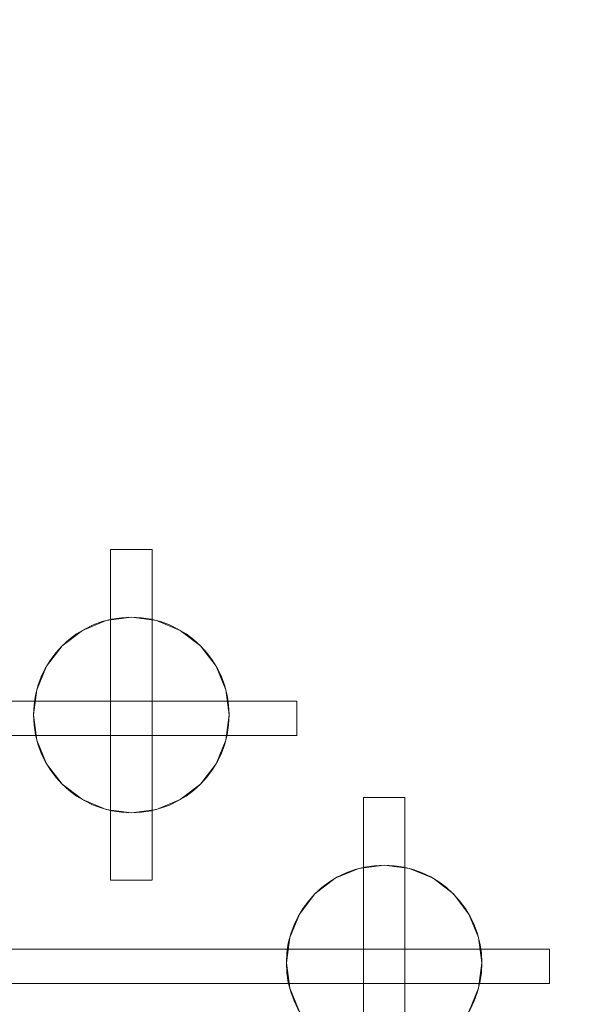
# Model space of a CAD drawing. Units: inches. Extents: x 2696 to 3240, y 1564 to 2310.
# Tile 9 of 76: x 2898.411 to 2903.397, y 1643.56 to 1652.487. Entities that reach past the tile are written whole.
import ezdxf

# ---------------------------------------------------------------- set-up
doc = ezdxf.new("R2010")
doc.units = ezdxf.units.IN
for name, color, linetype, lineweight in [('A-ANNO-DIMS', 3, 'Continuous', 18), ('A-FLOR-FIXT', 8, 'Continuous', 18), ('A-FURN', 251, 'Continuous', 13)]:
    doc.layers.add(name, color=color, linetype=linetype, lineweight=lineweight)
doc.layers.add('FURNITURE', color=250, linetype='Continuous')
doc.styles.add('TIMES NEW', font='times.ttf')
doc.dimstyles.new('Siddhuu', dxfattribs={"dimtxt": 6, "dimasz": 2.5, "dimexe": 1.25, "dimexo": 0.625, "dimtad": 1, "dimdec": 1, "dimlunit": 4, "dimtxsty": 'TIMES NEW', "dimcen": 2.5, "dimclrd": 256, "dimclre": 1, "dimclrt": 7, "dimadec": 0, "dimazin": 0, "dimtfac": 1, "dimtdec": 1, "dimtmove": 0, "dimatfit": 3, "dimfxl": 1, "dimtolj": 1, "dimlwd": -1, "dimarcsym": 0})

# ---------------------------------------------------------------- blocks, each defined once
blk = doc.blocks.new('A$C1af1f523')
at = {"layer": 'A-FURN'}
for p, q in [((-2.9003, 3.9351), (-2.9003, 0.9365)), ((-2.9003, 3.9351, 0.5), (-2.9003, 0.9365, 0.5)), ((-2.9003, 3.9351), (-2.9003, 3.9351, 0.5)), ((-2.5253, 3.9351), (-2.9003, 3.9351)), ((-2.5253, 3.9351, 0.5), (-2.9003, 3.9351, 0.5)), ((-2.5253, 3.9351), (-2.5253, 0.9365)), ((-2.5253, 3.9351, 0.5), (-2.5253, 0.9365, 0.5)), ((-2.5253, 3.9351), (-2.5253, 3.9351, 0.5)), ((-2.7128, 3.3215), (-2.7128, 3.3215, 0.5)), ((-2.9421, 3.2913), (-2.9421, 3.2913, 0.5)), ((-2.4835, 3.2913), (-2.4835, 3.2913, 0.5)), ((-3.1558, 3.2028), (-3.1558, 3.2028, 0.5)), ((-2.2698, 3.2028), (-2.2698, 3.2028, 0.5)), ((-3.3393, 3.062), (-3.3393, 3.062, 0.5)), ((-2.0863, 3.062), (-2.0863, 3.062, 0.5)), ((-3.4801, 2.8785), (-3.4801, 2.8785, 0.5)), ((-1.9455, 2.8785), (-1.9455, 2.8785, 0.5)), ((-3.5686, 2.6648), (-3.5686, 2.6648, 0.5)), ((-1.857, 2.6648), (-1.857, 2.6648, 0.5)), ((0, 2.5605), (-4.2116, 2.5605)), ((0, 2.5605, 0.5), (-4.2116, 2.5605, 0.5)), ((-4.2116, 2.5605), (-4.2116, 2.5605, 0.5)), ((-4.2116, 2.5594), (-4.2116, 2.248)), ((-4.2116, 2.5594, 0.5), (-4.2116, 2.248, 0.5)), ((-4.2116, 2.5594), (-4.2116, 2.5594, 0.5)), ((-3.5988, 2.4355), (-3.5988, 2.4355, 0.5)), ((-1.8268, 2.4355), (-1.8268, 2.4355, 0.5)), ((0, 2.248), (-4.2116, 2.248)), ((0, 2.248, 0.5), (-4.2116, 2.248, 0.5)), ((-4.2116, 2.248), (-4.2116, 2.248, 0.5)), ((-4.2116, 2.248), (-4.2116, 2.2469)), ((-4.2116, 2.248, 0.5), (-4.2116, 2.2469, 0.5)), ((-4.2116, 2.2469), (-4.2116, 2.2469, 0.5)), ((-3.5686, 2.2061), (-3.5686, 2.2061, 0.5)), ((-1.857, 2.2061), (-1.857, 2.2061, 0.5)), ((-3.4801, 1.9924), (-3.4801, 1.9924, 0.5)), ((-1.9455, 1.9924), (-1.9455, 1.9924, 0.5)), ((-3.3393, 1.8089), (-3.3393, 1.8089, 0.5)), ((-2.0863, 1.8089), (-2.0863, 1.8089, 0.5)), ((-4.8156, 1.6871), (-5.1906, 1.6871)), ((-4.8156, 1.6871, 0.5), (-5.1906, 1.6871, 0.5)), ((-5.1906, 1.6871), (-5.1906, 1.6871, 0.5)), ((-5.1906, 1.6871), (-5.1901, -1.3115)), ((-5.1906, 1.6871, 0.5), (-5.1901, -1.3115, 0.5)), ((-4.8156, 1.6871), (-4.8156, 1.6871, 0.5)), ((-4.8156, 1.6871), (-4.8151, -1.3115)), ((-4.8156, 1.6871, 0.5), (-4.8151, -1.3115, 0.5)), ((-3.1558, 1.6681), (-3.1558, 1.6681, 0.5)), ((-2.2698, 1.6681), (-2.2698, 1.6681, 0.5)), ((-2.9421, 1.5796), (-2.9421, 1.5796, 0.5)), ((-2.7128, 1.5494), (-2.7128, 1.5494, 0.5)), ((-2.4835, 1.5796), (-2.4835, 1.5796, 0.5)), ((-5.0026, 1.0735), (-5.0026, 1.0735, 0.5)), ((-5.232, 1.0433), (-5.232, 1.0433, 0.5)), ((-4.7733, 1.0433), (-4.7733, 1.0433, 0.5)), ((-5.4457, 0.9548), (-5.4457, 0.9548, 0.5)), ((-4.5596, 0.9548), (-4.5596, 0.9548, 0.5)), ((-2.9003, 0.9365), (-2.9003, 0.9365, 0.5)), ((-2.5253, 0.9365), (-2.8979, 0.9365)), ((-2.5253, 0.9365, 0.5), (-2.8979, 0.9365, 0.5)), ((-2.8979, 0.9365), (-2.8979, 0.9365, 0.5)), ((-2.5253, 0.9365), (-2.5253, 0.9365, 0.5)), ((-5.6292, 0.814), (-5.6292, 0.814, 0.5)), ((-4.3761, 0.814), (-4.3761, 0.814, 0.5)), ((-5.77, 0.6305), (-5.77, 0.6305, 0.5)), ((-4.2353, 0.6305), (-4.2353, 0.6305, 0.5)), ((-5.8585, 0.4168), (-5.8585, 0.4168, 0.5)), ((-4.1468, 0.4168), (-4.1468, 0.4168, 0.5)), ((0, 0.3125), (-6.5015, 0.3125)), ((0, 0.3125, 0.5), (-6.5015, 0.3125, 0.5)), ((-6.5015, 0.3125), (-6.5015, 0.3125, 0.5)), ((-6.5015, 0.3114), (-6.5015, 0)), ((-6.5015, 0.3114, 0.5), (-6.5015, 0, 0.5)), ((-6.5015, 0.3114), (-6.5015, 0.3114, 0.5)), ((-5.8887, 0.1875), (-5.8887, 0.1875, 0.5)), ((-4.1166, 0.1875), (-4.1166, 0.1875, 0.5)), ((0, 0), (-6.5015, 0)), ((0, 0, 0.5), (-6.5015, 0, 0.5)), ((-6.5015, 0), (-6.5015, 0, 0.5)), ((-6.5015, 0), (-6.5015, -0.0011)), ((-6.5015, 0, 0.5), (-6.5015, -0.0011, 0.5)), ((-6.5015, -0.0011), (-6.5015, -0.0011, 0.5)), ((-5.8585, -0.0418), (-5.8585, -0.0418, 0.5)), ((-4.1468, -0.0418), (-4.1468, -0.0418, 0.5)), ((-5.77, -0.2555), (-5.77, -0.2555, 0.5)), ((-4.2353, -0.2555), (-4.2353, -0.2555, 0.5)), ((-5.6292, -0.439), (-5.6292, -0.439, 0.5)), ((-4.3761, -0.439), (-4.3761, -0.439, 0.5)), ((-5.4457, -0.5798), (-5.4457, -0.5798, 0.5)), ((-4.5596, -0.5798), (-4.5596, -0.5798, 0.5)), ((-2.898, -0.5642), (-2.898, -3.5628)), ((-2.898, -0.5642, 0.5), (-2.898, -3.5628, 0.5)), ((-2.898, -0.5642), (-2.898, -0.5642, 0.5)), ((-2.523, -0.5642), (-2.898, -0.5642)), ((-2.523, -0.5642, 0.5), (-2.898, -0.5642, 0.5)), ((-2.523, -0.5642), (-2.523, -3.5628)), ((-2.523, -0.5642, 0.5), (-2.523, -3.5628, 0.5)), ((-2.523, -0.5642), (-2.523, -0.5642, 0.5)), ((-5.232, -0.6683), (-5.232, -0.6683, 0.5)), ((-5.0026, -0.6985), (-5.0026, -0.6985, 0.5)), ((-4.7733, -0.6683), (-4.7733, -0.6683, 0.5)), ((-2.9398, -1.208), (-2.9398, -1.208, 0.5)), ((-2.7105, -1.1778), (-2.7105, -1.1778, 0.5)), ((-2.4812, -1.208), (-2.4812, -1.208, 0.5)), ((-5.1901, -1.3115), (-5.1901, -1.3115, 0.5)), ((-4.8151, -1.3115), (-5.1878, -1.3115)), ((-4.8151, -1.3115, 0.5), (-5.1878, -1.3115, 0.5)), ((-5.1878, -1.3115), (-5.1878, -1.3115, 0.5)), ((-4.8151, -1.3115), (-4.8151, -1.3115, 0.5)), ((-3.1535, -1.2965), (-3.1535, -1.2965, 0.5)), ((-2.2675, -1.2965), (-2.2675, -1.2965, 0.5)), ((-3.337, -1.4373), (-3.337, -1.4373, 0.5)), ((-2.084, -1.4373), (-2.084, -1.4373, 0.5)), ((-3.4778, -1.6208), (-3.4778, -1.6208, 0.5)), ((-1.9432, -1.6208), (-1.9432, -1.6208, 0.5)), ((-3.5664, -1.8345), (-3.5664, -1.8345, 0.5)), ((-1.8547, -1.8345), (-1.8547, -1.8345, 0.5)), ((0, -1.9388), (-4.2094, -1.9388)), ((0, -1.9388, 0.5), (-4.2094, -1.9388, 0.5)), ((-4.2094, -1.9388), (-4.2094, -1.9388, 0.5)), ((-4.2094, -1.9399), (-4.2094, -2.2513)), ((-4.2094, -1.9399, 0.5), (-4.2094, -2.2513, 0.5)), ((-4.2094, -1.9399), (-4.2094, -1.9399, 0.5)), ((-3.5965, -2.0638), (-3.5965, -2.0638, 0.5)), ((-1.8245, -2.0638), (-1.8245, -2.0638, 0.5)), ((0, -2.2513), (-4.2094, -2.2513)), ((0, -2.2513, 0.5), (-4.2094, -2.2513, 0.5)), ((-4.2094, -2.2513), (-4.2094, -2.2513, 0.5)), ((-4.2094, -2.2513), (-4.2094, -2.2524)), ((-4.2094, -2.2513, 0.5), (-4.2094, -2.2524, 0.5)), ((-4.2094, -2.2524), (-4.2094, -2.2524, 0.5)), ((-3.5664, -2.2931), (-3.5664, -2.2931, 0.5)), ((-1.8547, -2.2931), (-1.8547, -2.2931, 0.5)), ((-3.4778, -2.5068), (-3.4778, -2.5068, 0.5)), ((-1.9432, -2.5068), (-1.9432, -2.5068, 0.5)), ((-3.337, -2.6903), (-3.337, -2.6903, 0.5)), ((-2.084, -2.6903), (-2.084, -2.6903, 0.5)), ((-3.1535, -2.8311), (-3.1535, -2.8311, 0.5)), ((-2.2675, -2.8311), (-2.2675, -2.8311, 0.5)), ((-2.9398, -2.9196), (-2.9398, -2.9196, 0.5)), ((-2.4812, -2.9196), (-2.4812, -2.9196, 0.5)), ((-2.7105, -2.9498), (-2.7105, -2.9498, 0.5)), ((-2.898, -3.5628), (-2.898, -3.5628, 0.5)), ((-2.523, -3.5628), (-2.8956, -3.5628)), ((-2.523, -3.5628, 0.5), (-2.8956, -3.5628, 0.5)), ((-2.8956, -3.5628), (-2.8956, -3.5628, 0.5)), ((-2.523, -3.5628), (-2.523, -3.5628, 0.5))]:
    blk.add_line(p, q, dxfattribs=at)
for centre in [(-2.7128, 2.4355), (-2.7128, 2.4355, 0.5), (-5.0026, 0.1875), (-5.0026, 0.1875, 0.5), (-2.7105, -2.0638), (-2.7105, -2.0638, 0.5)]:
    blk.add_circle(centre, 0.886, dxfattribs=at)
at = {"layer": 'FURNITURE'}
for p, q in [((0, 2.5605), (0, 2.5605, 0.5)), ((0, 2.248), (0, 2.248, 0.5)), ((0, 0.3125), (0, 0.3125, 0.5)), ((0, 0), (0, 0, 0.5)), ((0, -1.9388), (0, -1.9388, 0.5)), ((0, -2.2513), (0, -2.2513, 0.5))]:
    blk.add_line(p, q, dxfattribs=at)
at = {"layer": 'A-FURN'}
mesh = blk.add_polyface(dxfattribs=at)
corners = [(-2.9003, 0.9365, 0.5), (-2.9003, 3.9351), (-2.9003, 0.9365), (-2.9003, 3.9351, 0.5)]
mesh.append_faces([[corners[k] for k in face] for face in [(2, 1, 0), (3, 0, 1)]], dxfattribs={"vtx1": -1})
mesh = blk.add_polyface(dxfattribs=at)
corners = [(-2.5253, 3.9351, 0.5), (-2.9003, 3.9351), (-2.9003, 3.9351, 0.5), (-2.5253, 3.9351)]
mesh.append_faces([[corners[k] for k in face] for face in [(2, 1, 0), (3, 0, 1)]], dxfattribs={"vtx1": -1})
mesh = blk.add_polyface(dxfattribs=at)
corners = [(-2.5253, 0.9365, 0.5), (-2.5253, 3.9351), (-2.5253, 0.9365), (-2.5253, 3.9351, 0.5)]
mesh.append_faces([[corners[k] for k in face] for face in [(2, 1, 0), (3, 0, 1)]], dxfattribs={"vtx1": -1})
mesh = blk.add_polyface(dxfattribs=at)
corners = [(-2.7128, 3.3215), (-2.9421, 3.2913, 0.5), (-2.9421, 3.2913), (-2.7128, 3.3215, 0.5)]
mesh.append_faces([[corners[k] for k in face] for face in [(2, 1, 0), (3, 0, 1)]], dxfattribs={"vtx1": -1})
mesh = blk.add_polyface(dxfattribs=at)
corners = [(-2.4835, 3.2913), (-2.7128, 3.3215, 0.5), (-2.7128, 3.3215), (-2.4835, 3.2913, 0.5)]
mesh.append_faces([[corners[k] for k in face] for face in [(2, 1, 0), (3, 0, 1)]], dxfattribs={"vtx1": -1})
mesh = blk.add_polyface(dxfattribs=at)
corners = [(-2.9421, 3.2913), (-3.1558, 3.2028, 0.5), (-3.1558, 3.2028), (-2.9421, 3.2913, 0.5)]
mesh.append_faces([[corners[k] for k in face] for face in [(2, 1, 0), (3, 0, 1)]], dxfattribs={"vtx1": -1})
mesh = blk.add_polyface(dxfattribs=at)
corners = [(-2.2698, 3.2028), (-2.4835, 3.2913, 0.5), (-2.4835, 3.2913), (-2.2698, 3.2028, 0.5)]
mesh.append_faces([[corners[k] for k in face] for face in [(2, 1, 0), (3, 0, 1)]], dxfattribs={"vtx1": -1})
mesh = blk.add_polyface(dxfattribs=at)
corners = [(-3.1558, 3.2028), (-3.3393, 3.062, 0.5), (-3.3393, 3.062), (-3.1558, 3.2028, 0.5)]
mesh.append_faces([[corners[k] for k in face] for face in [(2, 1, 0), (3, 0, 1)]], dxfattribs={"vtx1": -1})
mesh = blk.add_polyface(dxfattribs=at)
corners = [(-2.0863, 3.062), (-2.2698, 3.2028, 0.5), (-2.2698, 3.2028), (-2.0863, 3.062, 0.5)]
mesh.append_faces([[corners[k] for k in face] for face in [(2, 1, 0), (3, 0, 1)]], dxfattribs={"vtx1": -1})
mesh = blk.add_polyface(dxfattribs=at)
corners = [(-3.3393, 3.062, 0.5), (-3.4801, 2.8785), (-3.3393, 3.062), (-3.4801, 2.8785, 0.5)]
mesh.append_faces([[corners[k] for k in face] for face in [(2, 1, 0), (3, 0, 1)]], dxfattribs={"vtx1": -1})
mesh = blk.add_polyface(dxfattribs=at)
corners = [(-1.9455, 2.8785, 0.5), (-2.0863, 3.062), (-1.9455, 2.8785), (-2.0863, 3.062, 0.5)]
mesh.append_faces([[corners[k] for k in face] for face in [(2, 1, 0), (3, 0, 1)]], dxfattribs={"vtx1": -1})
mesh = blk.add_polyface(dxfattribs=at)
corners = [(-3.4801, 2.8785, 0.5), (-3.5686, 2.6648), (-3.4801, 2.8785), (-3.5686, 2.6648, 0.5)]
mesh.append_faces([[corners[k] for k in face] for face in [(2, 1, 0), (3, 0, 1)]], dxfattribs={"vtx1": -1})
mesh = blk.add_polyface(dxfattribs=at)
corners = [(-1.857, 2.6648, 0.5), (-1.9455, 2.8785), (-1.857, 2.6648), (-1.9455, 2.8785, 0.5)]
mesh.append_faces([[corners[k] for k in face] for face in [(2, 1, 0), (3, 0, 1)]], dxfattribs={"vtx1": -1})
mesh = blk.add_polyface(dxfattribs=at)
corners = [(-3.5686, 2.6648, 0.5), (-3.5988, 2.4355), (-3.5686, 2.6648), (-3.5988, 2.4355, 0.5)]
mesh.append_faces([[corners[k] for k in face] for face in [(2, 1, 0), (3, 0, 1)]], dxfattribs={"vtx1": -1})
mesh = blk.add_polyface(dxfattribs=at)
corners = [(-1.8268, 2.4355, 0.5), (-1.857, 2.6648), (-1.8268, 2.4355), (-1.857, 2.6648, 0.5)]
mesh.append_faces([[corners[k] for k in face] for face in [(2, 1, 0), (3, 0, 1)]], dxfattribs={"vtx1": -1})
mesh = blk.add_polyface(dxfattribs=at)
corners = [(0, 2.5605, 0.5), (-4.2116, 2.5605), (-4.2116, 2.5605, 0.5), (0, 2.5605)]
mesh.append_faces([[corners[k] for k in face] for face in [(2, 1, 0), (3, 0, 1)]], dxfattribs={"vtx1": -1})
mesh = blk.add_polyface(dxfattribs=at)
corners = [(-4.2116, 2.2469, 0.5), (-4.2116, 2.248), (-4.2116, 2.2469), (-4.2116, 2.5594), (-4.2116, 2.5594, 0.5), (-4.2116, 2.248, 0.5)]
mesh.append_faces([[corners[k] for k in face] for face in [(3, 0, 1), (4, 0, 3)]], dxfattribs={"vtx0": -1, "vtx1": -1})
mesh.append_faces([[corners[k] for k in face] for face in [(2, 1, 0), (5, 0, 4)]], dxfattribs={"vtx1": -1})
mesh = blk.add_polyface(dxfattribs=at)
corners = [(-3.5988, 2.4355, 0.5), (-3.5686, 2.2061), (-3.5988, 2.4355), (-3.5686, 2.2061, 0.5)]
mesh.append_faces([[corners[k] for k in face] for face in [(2, 1, 0), (3, 0, 1)]], dxfattribs={"vtx1": -1})
mesh = blk.add_polyface(dxfattribs=at)
corners = [(-1.857, 2.2061, 0.5), (-1.8268, 2.4355), (-1.857, 2.2061), (-1.8268, 2.4355, 0.5)]
mesh.append_faces([[corners[k] for k in face] for face in [(2, 1, 0), (3, 0, 1)]], dxfattribs={"vtx1": -1})
mesh = blk.add_polyface(dxfattribs=at)
corners = [(0, 2.248, 0.5), (-4.2116, 2.248), (-4.2116, 2.248, 0.5), (0, 2.248)]
mesh.append_faces([[corners[k] for k in face] for face in [(2, 1, 0), (3, 0, 1)]], dxfattribs={"vtx1": -1})
mesh = blk.add_polyface(dxfattribs=at)
corners = [(-3.5686, 2.2061, 0.5), (-3.4801, 1.9924), (-3.5686, 2.2061), (-3.4801, 1.9924, 0.5)]
mesh.append_faces([[corners[k] for k in face] for face in [(2, 1, 0), (3, 0, 1)]], dxfattribs={"vtx1": -1})
mesh = blk.add_polyface(dxfattribs=at)
corners = [(-1.9455, 1.9924, 0.5), (-1.857, 2.2061), (-1.9455, 1.9924), (-1.857, 2.2061, 0.5)]
mesh.append_faces([[corners[k] for k in face] for face in [(2, 1, 0), (3, 0, 1)]], dxfattribs={"vtx1": -1})
mesh = blk.add_polyface(dxfattribs=at)
corners = [(-3.4801, 1.9924, 0.5), (-3.3393, 1.8089), (-3.4801, 1.9924), (-3.3393, 1.8089, 0.5)]
mesh.append_faces([[corners[k] for k in face] for face in [(2, 1, 0), (3, 0, 1)]], dxfattribs={"vtx1": -1})
mesh = blk.add_polyface(dxfattribs=at)
corners = [(-2.0863, 1.8089, 0.5), (-1.9455, 1.9924), (-2.0863, 1.8089), (-1.9455, 1.9924, 0.5)]
mesh.append_faces([[corners[k] for k in face] for face in [(2, 1, 0), (3, 0, 1)]], dxfattribs={"vtx1": -1})
mesh = blk.add_polyface(dxfattribs=at)
corners = [(-3.1558, 1.6681, 0.5), (-3.3393, 1.8089), (-3.3393, 1.8089, 0.5), (-3.1558, 1.6681)]
mesh.append_faces([[corners[k] for k in face] for face in [(2, 1, 0), (3, 0, 1)]], dxfattribs={"vtx1": -1})
mesh = blk.add_polyface(dxfattribs=at)
corners = [(-2.0863, 1.8089, 0.5), (-2.2698, 1.6681), (-2.2698, 1.6681, 0.5), (-2.0863, 1.8089)]
mesh.append_faces([[corners[k] for k in face] for face in [(2, 1, 0), (3, 0, 1)]], dxfattribs={"vtx1": -1})
mesh = blk.add_polyface(dxfattribs=at)
corners = [(-4.8156, 1.6871, 0.5), (-5.1906, 1.6871), (-5.1906, 1.6871, 0.5), (-4.8156, 1.6871)]
mesh.append_faces([[corners[k] for k in face] for face in [(2, 1, 0), (3, 0, 1)]], dxfattribs={"vtx1": -1})
mesh = blk.add_polyface(dxfattribs=at)
corners = [(-5.1901, -1.3115, 0.5), (-5.1906, 1.6871), (-5.1901, -1.3115), (-5.1906, 1.6871, 0.5)]
mesh.append_faces([[corners[k] for k in face] for face in [(2, 1, 0), (3, 0, 1)]], dxfattribs={"vtx1": -1})
mesh = blk.add_polyface(dxfattribs=at)
corners = [(-4.8151, -1.3115, 0.5), (-4.8156, 1.6871), (-4.8151, -1.3115), (-4.8156, 1.6871, 0.5)]
mesh.append_faces([[corners[k] for k in face] for face in [(2, 1, 0), (3, 0, 1)]], dxfattribs={"vtx1": -1})
mesh = blk.add_polyface(dxfattribs=at)
corners = [(-2.9421, 1.5796, 0.5), (-3.1558, 1.6681), (-3.1558, 1.6681, 0.5), (-2.9421, 1.5796)]
mesh.append_faces([[corners[k] for k in face] for face in [(2, 1, 0), (3, 0, 1)]], dxfattribs={"vtx1": -1})
mesh = blk.add_polyface(dxfattribs=at)
corners = [(-2.2698, 1.6681, 0.5), (-2.4835, 1.5796), (-2.4835, 1.5796, 0.5), (-2.2698, 1.6681)]
mesh.append_faces([[corners[k] for k in face] for face in [(2, 1, 0), (3, 0, 1)]], dxfattribs={"vtx1": -1})
mesh = blk.add_polyface(dxfattribs=at)
corners = [(-2.7128, 1.5494, 0.5), (-2.9421, 1.5796), (-2.9421, 1.5796, 0.5), (-2.7128, 1.5494)]
mesh.append_faces([[corners[k] for k in face] for face in [(2, 1, 0), (3, 0, 1)]], dxfattribs={"vtx1": -1})
mesh = blk.add_polyface(dxfattribs=at)
corners = [(-2.4835, 1.5796, 0.5), (-2.7128, 1.5494), (-2.7128, 1.5494, 0.5), (-2.4835, 1.5796)]
mesh.append_faces([[corners[k] for k in face] for face in [(2, 1, 0), (3, 0, 1)]], dxfattribs={"vtx1": -1})
mesh = blk.add_polyface(dxfattribs=at)
corners = [(-5.0026, 1.0735), (-5.232, 1.0433, 0.5), (-5.232, 1.0433), (-5.0026, 1.0735, 0.5)]
mesh.append_faces([[corners[k] for k in face] for face in [(2, 1, 0), (3, 0, 1)]], dxfattribs={"vtx1": -1})
mesh = blk.add_polyface(dxfattribs=at)
corners = [(-4.7733, 1.0433), (-5.0026, 1.0735, 0.5), (-5.0026, 1.0735), (-4.7733, 1.0433, 0.5)]
mesh.append_faces([[corners[k] for k in face] for face in [(2, 1, 0), (3, 0, 1)]], dxfattribs={"vtx1": -1})
mesh = blk.add_polyface(dxfattribs=at)
corners = [(-5.232, 1.0433), (-5.4457, 0.9548, 0.5), (-5.4457, 0.9548), (-5.232, 1.0433, 0.5)]
mesh.append_faces([[corners[k] for k in face] for face in [(2, 1, 0), (3, 0, 1)]], dxfattribs={"vtx1": -1})
mesh = blk.add_polyface(dxfattribs=at)
corners = [(-4.5596, 0.9548), (-4.7733, 1.0433, 0.5), (-4.7733, 1.0433), (-4.5596, 0.9548, 0.5)]
mesh.append_faces([[corners[k] for k in face] for face in [(2, 1, 0), (3, 0, 1)]], dxfattribs={"vtx1": -1})
mesh = blk.add_polyface(dxfattribs=at)
corners = [(-5.4457, 0.9548), (-5.6292, 0.814, 0.5), (-5.6292, 0.814), (-5.4457, 0.9548, 0.5)]
mesh.append_faces([[corners[k] for k in face] for face in [(2, 1, 0), (3, 0, 1)]], dxfattribs={"vtx1": -1})
mesh = blk.add_polyface(dxfattribs=at)
corners = [(-4.3761, 0.814), (-4.5596, 0.9548, 0.5), (-4.5596, 0.9548), (-4.3761, 0.814, 0.5)]
mesh.append_faces([[corners[k] for k in face] for face in [(2, 1, 0), (3, 0, 1)]], dxfattribs={"vtx1": -1})
mesh = blk.add_polyface(dxfattribs=at)
corners = [(-2.5253, 0.9365, 0.5), (-2.8979, 0.9365), (-2.8979, 0.9365, 0.5), (-2.5253, 0.9365)]
mesh.append_faces([[corners[k] for k in face] for face in [(2, 1, 0), (3, 0, 1)]], dxfattribs={"vtx1": -1})
mesh = blk.add_polyface(dxfattribs=at)
corners = [(-5.6292, 0.814, 0.5), (-5.77, 0.6305), (-5.6292, 0.814), (-5.77, 0.6305, 0.5)]
mesh.append_faces([[corners[k] for k in face] for face in [(2, 1, 0), (3, 0, 1)]], dxfattribs={"vtx1": -1})
mesh = blk.add_polyface(dxfattribs=at)
corners = [(-4.2353, 0.6305, 0.5), (-4.3761, 0.814), (-4.2353, 0.6305), (-4.3761, 0.814, 0.5)]
mesh.append_faces([[corners[k] for k in face] for face in [(2, 1, 0), (3, 0, 1)]], dxfattribs={"vtx1": -1})
mesh = blk.add_polyface(dxfattribs=at)
corners = [(-5.77, 0.6305, 0.5), (-5.8585, 0.4168), (-5.77, 0.6305), (-5.8585, 0.4168, 0.5)]
mesh.append_faces([[corners[k] for k in face] for face in [(2, 1, 0), (3, 0, 1)]], dxfattribs={"vtx1": -1})
mesh = blk.add_polyface(dxfattribs=at)
corners = [(-4.1468, 0.4168, 0.5), (-4.2353, 0.6305), (-4.1468, 0.4168), (-4.2353, 0.6305, 0.5)]
mesh.append_faces([[corners[k] for k in face] for face in [(2, 1, 0), (3, 0, 1)]], dxfattribs={"vtx1": -1})
mesh = blk.add_polyface(dxfattribs=at)
corners = [(-5.8585, 0.4168, 0.5), (-5.8887, 0.1875), (-5.8585, 0.4168), (-5.8887, 0.1875, 0.5)]
mesh.append_faces([[corners[k] for k in face] for face in [(2, 1, 0), (3, 0, 1)]], dxfattribs={"vtx1": -1})
mesh = blk.add_polyface(dxfattribs=at)
corners = [(-4.1166, 0.1875, 0.5), (-4.1468, 0.4168), (-4.1166, 0.1875), (-4.1468, 0.4168, 0.5)]
mesh.append_faces([[corners[k] for k in face] for face in [(2, 1, 0), (3, 0, 1)]], dxfattribs={"vtx1": -1})
mesh = blk.add_polyface(dxfattribs=at)
corners = [(0, 0.3125, 0.5), (-6.5015, 0.3125), (-6.5015, 0.3125, 0.5), (0, 0.3125)]
mesh.append_faces([[corners[k] for k in face] for face in [(2, 1, 0), (3, 0, 1)]], dxfattribs={"vtx1": -1})
mesh = blk.add_polyface(dxfattribs=at)
corners = [(-6.5015, -0.0011, 0.5), (-6.5015, 0), (-6.5015, -0.0011), (-6.5015, 0.3114), (-6.5015, 0.3114, 0.5), (-6.5015, 0, 0.5)]
mesh.append_faces([[corners[k] for k in face] for face in [(3, 0, 1), (4, 0, 3)]], dxfattribs={"vtx0": -1, "vtx1": -1})
mesh.append_faces([[corners[k] for k in face] for face in [(2, 1, 0), (5, 0, 4)]], dxfattribs={"vtx1": -1})
mesh = blk.add_polyface(dxfattribs=at)
corners = [(-5.8887, 0.1875, 0.5), (-5.8585, -0.0418), (-5.8887, 0.1875), (-5.8585, -0.0418, 0.5)]
mesh.append_faces([[corners[k] for k in face] for face in [(2, 1, 0), (3, 0, 1)]], dxfattribs={"vtx1": -1})
mesh = blk.add_polyface(dxfattribs=at)
corners = [(-4.1468, -0.0418, 0.5), (-4.1166, 0.1875), (-4.1468, -0.0418), (-4.1166, 0.1875, 0.5)]
mesh.append_faces([[corners[k] for k in face] for face in [(2, 1, 0), (3, 0, 1)]], dxfattribs={"vtx1": -1})
mesh = blk.add_polyface(dxfattribs=at)
corners = [(0, 0, 0.5), (-6.5015, 0), (-6.5015, 0, 0.5), (0, 0)]
mesh.append_faces([[corners[k] for k in face] for face in [(2, 1, 0), (3, 0, 1)]], dxfattribs={"vtx1": -1})
mesh = blk.add_polyface(dxfattribs=at)
corners = [(-5.8585, -0.0418, 0.5), (-5.77, -0.2555), (-5.8585, -0.0418), (-5.77, -0.2555, 0.5)]
mesh.append_faces([[corners[k] for k in face] for face in [(2, 1, 0), (3, 0, 1)]], dxfattribs={"vtx1": -1})
mesh = blk.add_polyface(dxfattribs=at)
corners = [(-4.2353, -0.2555, 0.5), (-4.1468, -0.0418), (-4.2353, -0.2555), (-4.1468, -0.0418, 0.5)]
mesh.append_faces([[corners[k] for k in face] for face in [(2, 1, 0), (3, 0, 1)]], dxfattribs={"vtx1": -1})
mesh = blk.add_polyface(dxfattribs=at)
corners = [(-5.77, -0.2555, 0.5), (-5.6292, -0.439), (-5.77, -0.2555), (-5.6292, -0.439, 0.5)]
mesh.append_faces([[corners[k] for k in face] for face in [(2, 1, 0), (3, 0, 1)]], dxfattribs={"vtx1": -1})
mesh = blk.add_polyface(dxfattribs=at)
corners = [(-4.3761, -0.439, 0.5), (-4.2353, -0.2555), (-4.3761, -0.439), (-4.2353, -0.2555, 0.5)]
mesh.append_faces([[corners[k] for k in face] for face in [(2, 1, 0), (3, 0, 1)]], dxfattribs={"vtx1": -1})
mesh = blk.add_polyface(dxfattribs=at)
corners = [(-5.4457, -0.5798, 0.5), (-5.6292, -0.439), (-5.6292, -0.439, 0.5), (-5.4457, -0.5798)]
mesh.append_faces([[corners[k] for k in face] for face in [(2, 1, 0), (3, 0, 1)]], dxfattribs={"vtx1": -1})
mesh = blk.add_polyface(dxfattribs=at)
corners = [(-4.3761, -0.439, 0.5), (-4.5596, -0.5798), (-4.5596, -0.5798, 0.5), (-4.3761, -0.439)]
mesh.append_faces([[corners[k] for k in face] for face in [(2, 1, 0), (3, 0, 1)]], dxfattribs={"vtx1": -1})
mesh = blk.add_polyface(dxfattribs=at)
corners = [(-5.232, -0.6683, 0.5), (-5.4457, -0.5798), (-5.4457, -0.5798, 0.5), (-5.232, -0.6683)]
mesh.append_faces([[corners[k] for k in face] for face in [(2, 1, 0), (3, 0, 1)]], dxfattribs={"vtx1": -1})
mesh = blk.add_polyface(dxfattribs=at)
corners = [(-4.5596, -0.5798, 0.5), (-4.7733, -0.6683), (-4.7733, -0.6683, 0.5), (-4.5596, -0.5798)]
mesh.append_faces([[corners[k] for k in face] for face in [(2, 1, 0), (3, 0, 1)]], dxfattribs={"vtx1": -1})
mesh = blk.add_polyface(dxfattribs=at)
corners = [(-2.898, -3.5628, 0.5), (-2.898, -0.5642), (-2.898, -3.5628), (-2.898, -0.5642, 0.5)]
mesh.append_faces([[corners[k] for k in face] for face in [(2, 1, 0), (3, 0, 1)]], dxfattribs={"vtx1": -1})
mesh = blk.add_polyface(dxfattribs=at)
corners = [(-2.523, -0.5642, 0.5), (-2.898, -0.5642), (-2.898, -0.5642, 0.5), (-2.523, -0.5642)]
mesh.append_faces([[corners[k] for k in face] for face in [(2, 1, 0), (3, 0, 1)]], dxfattribs={"vtx1": -1})
mesh = blk.add_polyface(dxfattribs=at)
corners = [(-2.523, -3.5628, 0.5), (-2.523, -0.5642), (-2.523, -3.5628), (-2.523, -0.5642, 0.5)]
mesh.append_faces([[corners[k] for k in face] for face in [(2, 1, 0), (3, 0, 1)]], dxfattribs={"vtx1": -1})
mesh = blk.add_polyface(dxfattribs=at)
corners = [(-5.0026, -0.6985, 0.5), (-5.232, -0.6683), (-5.232, -0.6683, 0.5), (-5.0026, -0.6985)]
mesh.append_faces([[corners[k] for k in face] for face in [(2, 1, 0), (3, 0, 1)]], dxfattribs={"vtx1": -1})
mesh = blk.add_polyface(dxfattribs=at)
corners = [(-4.7733, -0.6683, 0.5), (-5.0026, -0.6985), (-5.0026, -0.6985, 0.5), (-4.7733, -0.6683)]
mesh.append_faces([[corners[k] for k in face] for face in [(2, 1, 0), (3, 0, 1)]], dxfattribs={"vtx1": -1})
mesh = blk.add_polyface(dxfattribs=at)
corners = [(-2.9398, -1.208), (-3.1535, -1.2965, 0.5), (-3.1535, -1.2965), (-2.9398, -1.208, 0.5)]
mesh.append_faces([[corners[k] for k in face] for face in [(2, 1, 0), (3, 0, 1)]], dxfattribs={"vtx1": -1})
mesh = blk.add_polyface(dxfattribs=at)
corners = [(-2.7105, -1.1778), (-2.9398, -1.208, 0.5), (-2.9398, -1.208), (-2.7105, -1.1778, 0.5)]
mesh.append_faces([[corners[k] for k in face] for face in [(2, 1, 0), (3, 0, 1)]], dxfattribs={"vtx1": -1})
mesh = blk.add_polyface(dxfattribs=at)
corners = [(-2.4812, -1.208), (-2.7105, -1.1778, 0.5), (-2.7105, -1.1778), (-2.4812, -1.208, 0.5)]
mesh.append_faces([[corners[k] for k in face] for face in [(2, 1, 0), (3, 0, 1)]], dxfattribs={"vtx1": -1})
mesh = blk.add_polyface(dxfattribs=at)
corners = [(-2.2675, -1.2965), (-2.4812, -1.208, 0.5), (-2.4812, -1.208), (-2.2675, -1.2965, 0.5)]
mesh.append_faces([[corners[k] for k in face] for face in [(2, 1, 0), (3, 0, 1)]], dxfattribs={"vtx1": -1})
mesh = blk.add_polyface(dxfattribs=at)
corners = [(-4.8151, -1.3115, 0.5), (-5.1878, -1.3115), (-5.1878, -1.3115, 0.5), (-4.8151, -1.3115)]
mesh.append_faces([[corners[k] for k in face] for face in [(2, 1, 0), (3, 0, 1)]], dxfattribs={"vtx1": -1})
mesh = blk.add_polyface(dxfattribs=at)
corners = [(-3.1535, -1.2965), (-3.337, -1.4373, 0.5), (-3.337, -1.4373), (-3.1535, -1.2965, 0.5)]
mesh.append_faces([[corners[k] for k in face] for face in [(2, 1, 0), (3, 0, 1)]], dxfattribs={"vtx1": -1})
mesh = blk.add_polyface(dxfattribs=at)
corners = [(-2.084, -1.4373), (-2.2675, -1.2965, 0.5), (-2.2675, -1.2965), (-2.084, -1.4373, 0.5)]
mesh.append_faces([[corners[k] for k in face] for face in [(2, 1, 0), (3, 0, 1)]], dxfattribs={"vtx1": -1})
mesh = blk.add_polyface(dxfattribs=at)
corners = [(-3.337, -1.4373, 0.5), (-3.4778, -1.6208), (-3.337, -1.4373), (-3.4778, -1.6208, 0.5)]
mesh.append_faces([[corners[k] for k in face] for face in [(2, 1, 0), (3, 0, 1)]], dxfattribs={"vtx1": -1})
mesh = blk.add_polyface(dxfattribs=at)
corners = [(-1.9432, -1.6208, 0.5), (-2.084, -1.4373), (-1.9432, -1.6208), (-2.084, -1.4373, 0.5)]
mesh.append_faces([[corners[k] for k in face] for face in [(2, 1, 0), (3, 0, 1)]], dxfattribs={"vtx1": -1})
mesh = blk.add_polyface(dxfattribs=at)
corners = [(-3.4778, -1.6208, 0.5), (-3.5664, -1.8345), (-3.4778, -1.6208), (-3.5664, -1.8345, 0.5)]
mesh.append_faces([[corners[k] for k in face] for face in [(2, 1, 0), (3, 0, 1)]], dxfattribs={"vtx1": -1})
mesh = blk.add_polyface(dxfattribs=at)
corners = [(-1.8547, -1.8345, 0.5), (-1.9432, -1.6208), (-1.8547, -1.8345), (-1.9432, -1.6208, 0.5)]
mesh.append_faces([[corners[k] for k in face] for face in [(2, 1, 0), (3, 0, 1)]], dxfattribs={"vtx1": -1})
mesh = blk.add_polyface(dxfattribs=at)
corners = [(-3.5664, -1.8345, 0.5), (-3.5965, -2.0638), (-3.5664, -1.8345), (-3.5965, -2.0638, 0.5)]
mesh.append_faces([[corners[k] for k in face] for face in [(2, 1, 0), (3, 0, 1)]], dxfattribs={"vtx1": -1})
mesh = blk.add_polyface(dxfattribs=at)
corners = [(-1.8245, -2.0638, 0.5), (-1.8547, -1.8345), (-1.8245, -2.0638), (-1.8547, -1.8345, 0.5)]
mesh.append_faces([[corners[k] for k in face] for face in [(2, 1, 0), (3, 0, 1)]], dxfattribs={"vtx1": -1})
mesh = blk.add_polyface(dxfattribs=at)
corners = [(0, -1.9388, 0.5), (-4.2094, -1.9388), (-4.2094, -1.9388, 0.5), (0, -1.9388)]
mesh.append_faces([[corners[k] for k in face] for face in [(2, 1, 0), (3, 0, 1)]], dxfattribs={"vtx1": -1})
mesh = blk.add_polyface(dxfattribs=at)
corners = [(-4.2094, -2.2524, 0.5), (-4.2094, -2.2513), (-4.2094, -2.2524), (-4.2094, -1.9399), (-4.2094, -1.9399, 0.5), (-4.2094, -2.2513, 0.5)]
mesh.append_faces([[corners[k] for k in face] for face in [(3, 0, 1), (4, 0, 3)]], dxfattribs={"vtx0": -1, "vtx1": -1})
mesh.append_faces([[corners[k] for k in face] for face in [(2, 1, 0), (5, 0, 4)]], dxfattribs={"vtx1": -1})
mesh = blk.add_polyface(dxfattribs=at)
corners = [(-3.5965, -2.0638, 0.5), (-3.5664, -2.2931), (-3.5965, -2.0638), (-3.5664, -2.2931, 0.5)]
mesh.append_faces([[corners[k] for k in face] for face in [(2, 1, 0), (3, 0, 1)]], dxfattribs={"vtx1": -1})
mesh = blk.add_polyface(dxfattribs=at)
corners = [(-1.8547, -2.2931, 0.5), (-1.8245, -2.0638), (-1.8547, -2.2931), (-1.8245, -2.0638, 0.5)]
mesh.append_faces([[corners[k] for k in face] for face in [(2, 1, 0), (3, 0, 1)]], dxfattribs={"vtx1": -1})
mesh = blk.add_polyface(dxfattribs=at)
corners = [(0, -2.2513, 0.5), (-4.2094, -2.2513), (-4.2094, -2.2513, 0.5), (0, -2.2513)]
mesh.append_faces([[corners[k] for k in face] for face in [(2, 1, 0), (3, 0, 1)]], dxfattribs={"vtx1": -1})
mesh = blk.add_polyface(dxfattribs=at)
corners = [(-3.5664, -2.2931, 0.5), (-3.4778, -2.5068), (-3.5664, -2.2931), (-3.4778, -2.5068, 0.5)]
mesh.append_faces([[corners[k] for k in face] for face in [(2, 1, 0), (3, 0, 1)]], dxfattribs={"vtx1": -1})
mesh = blk.add_polyface(dxfattribs=at)
corners = [(-1.9432, -2.5068, 0.5), (-1.8547, -2.2931), (-1.9432, -2.5068), (-1.8547, -2.2931, 0.5)]
mesh.append_faces([[corners[k] for k in face] for face in [(2, 1, 0), (3, 0, 1)]], dxfattribs={"vtx1": -1})
mesh = blk.add_polyface(dxfattribs=at)
corners = [(-3.4778, -2.5068, 0.5), (-3.337, -2.6903), (-3.4778, -2.5068), (-3.337, -2.6903, 0.5)]
mesh.append_faces([[corners[k] for k in face] for face in [(2, 1, 0), (3, 0, 1)]], dxfattribs={"vtx1": -1})
mesh = blk.add_polyface(dxfattribs=at)
corners = [(-2.084, -2.6903, 0.5), (-1.9432, -2.5068), (-2.084, -2.6903), (-1.9432, -2.5068, 0.5)]
mesh.append_faces([[corners[k] for k in face] for face in [(2, 1, 0), (3, 0, 1)]], dxfattribs={"vtx1": -1})
mesh = blk.add_polyface(dxfattribs=at)
corners = [(-3.1535, -2.8311, 0.5), (-3.337, -2.6903), (-3.337, -2.6903, 0.5), (-3.1535, -2.8311)]
mesh.append_faces([[corners[k] for k in face] for face in [(2, 1, 0), (3, 0, 1)]], dxfattribs={"vtx1": -1})
mesh = blk.add_polyface(dxfattribs=at)
corners = [(-2.084, -2.6903, 0.5), (-2.2675, -2.8311), (-2.2675, -2.8311, 0.5), (-2.084, -2.6903)]
mesh.append_faces([[corners[k] for k in face] for face in [(2, 1, 0), (3, 0, 1)]], dxfattribs={"vtx1": -1})
mesh = blk.add_polyface(dxfattribs=at)
corners = [(-2.9398, -2.9196, 0.5), (-3.1535, -2.8311), (-3.1535, -2.8311, 0.5), (-2.9398, -2.9196)]
mesh.append_faces([[corners[k] for k in face] for face in [(2, 1, 0), (3, 0, 1)]], dxfattribs={"vtx1": -1})
mesh = blk.add_polyface(dxfattribs=at)
corners = [(-2.2675, -2.8311, 0.5), (-2.4812, -2.9196), (-2.4812, -2.9196, 0.5), (-2.2675, -2.8311)]
mesh.append_faces([[corners[k] for k in face] for face in [(2, 1, 0), (3, 0, 1)]], dxfattribs={"vtx1": -1})
mesh = blk.add_polyface(dxfattribs=at)
corners = [(-2.7105, -2.9498, 0.5), (-2.9398, -2.9196), (-2.9398, -2.9196, 0.5), (-2.7105, -2.9498)]
mesh.append_faces([[corners[k] for k in face] for face in [(2, 1, 0), (3, 0, 1)]], dxfattribs={"vtx1": -1})
mesh = blk.add_polyface(dxfattribs=at)
corners = [(-2.4812, -2.9196, 0.5), (-2.7105, -2.9498), (-2.7105, -2.9498, 0.5), (-2.4812, -2.9196)]
mesh.append_faces([[corners[k] for k in face] for face in [(2, 1, 0), (3, 0, 1)]], dxfattribs={"vtx1": -1})
mesh = blk.add_polyface(dxfattribs=at)
corners = [(-2.523, -3.5628, 0.5), (-2.8956, -3.5628), (-2.8956, -3.5628, 0.5), (-2.523, -3.5628)]
mesh.append_faces([[corners[k] for k in face] for face in [(2, 1, 0), (3, 0, 1)]], dxfattribs={"vtx1": -1})
blk = doc.blocks.new('*D57')
at = {"layer": 'A-ANNO-DIMS', "color": 1, "lineweight": -2, "transparency": 16777216}
for p, q in [((2754.6114, 2018.5761), (2754.6114, 1568.9511)), ((2956.7088, 2018.5761), (2956.7088, 1568.9511))]:
    blk.add_line(p, q, dxfattribs=at)
at = {"layer": 'A-ANNO-DIMS', "transparency": 16777216}
blk.add_line((2757.1114, 1570.2011), (2954.2088, 1570.2011), dxfattribs=at)
for points in [[(2757.1114, 1570.6178), (2757.1114, 1569.7844), (2754.6114, 1570.2011)], [(2954.2088, 1570.6178), (2954.2088, 1569.7844), (2956.7088, 1570.2011)]]:
    blk.add_solid(points, dxfattribs=at)
at = {"layer": 'Defpoints', "color": 0, "transparency": 16777216}
for p in [(2754.6114, 2019.2011), (2956.7088, 2019.2011), (2956.7088, 1570.2011)]:
    blk.add_point(p, dxfattribs=at)
at = {"layer": 'A-ANNO-DIMS', "color": 7, "transparency": 16777216, "insert": (2855.6601, 1573.878), "char_height": 6, "attachment_point": 5, "style": 'TIMES NEW'}
blk.add_mtext('\\A1;16\'-10"', dxfattribs=at)
blk = doc.blocks.new('*D69')
at = {"layer": 'A-ANNO-DIMS', "color": 1, "lineweight": -2, "transparency": 16777216}
for p, q in [((2841.889, 2261.5761), (2841.889, 1568.9511)), ((2905.9101, 2261.5761), (2905.9101, 1568.9511))]:
    blk.add_line(p, q, dxfattribs=at)
at = {"layer": 'A-ANNO-DIMS', "transparency": 16777216}
blk.add_line((2844.389, 1570.2011), (2903.4101, 1570.2011), dxfattribs=at)
for points in [[(2844.389, 1570.6178), (2844.389, 1569.7844), (2841.889, 1570.2011)], [(2903.4101, 1570.6178), (2903.4101, 1569.7844), (2905.9101, 1570.2011)]]:
    blk.add_solid(points, dxfattribs=at)
at = {"layer": 'Defpoints', "color": 0, "transparency": 16777216}
for p in [(2841.889, 2262.2011), (2905.9101, 2262.2011), (2905.9101, 1570.2011)]:
    blk.add_point(p, dxfattribs=at)
at = {"layer": 'A-ANNO-DIMS', "color": 7, "transparency": 16777216, "insert": (2873.8995, 1573.878), "char_height": 6, "attachment_point": 5, "style": 'TIMES NEW'}
blk.add_mtext('\\A1;5\'-4"', dxfattribs=at)

msp = doc.modelspace()

# ---------------------------------------------------------------- block references
at = {"layer": 'A-FLOR-FIXT', "xscale": -1}
msp.add_blockref('A$C1af1f523', (2896.7088, 1643.7478), dxfattribs=at)

# ---------------------------------------------------------------- dimensions: what is measured, and where the dimension line sits
at = {"layer": 'A-ANNO-DIMS'}
for base, p1, p2, picture, middle in [((2905.9101, 1570.2011), (2841.889, 2262.2011), (2905.9101, 2262.2011), '*D69', (2873.8995, 1573.878)), ((2956.7088, 1570.2011), (2754.6114, 2019.2011), (2956.7088, 2019.2011), '*D57', (2855.6601, 1573.878))]:
    dim = msp.add_linear_dim(base=base, p1=p1, p2=p2, dimstyle='Siddhuu', override={"dimdec": 1, "dimlfac": 1, "dimrnd": 0, "dimzin": 1, "dimdsep": 46, "dimlunit": 4, "dimfrac": 2}, dxfattribs=at)
    dim.commit()
    dim.dimension.update_dxf_attribs({"geometry": picture, "text_midpoint": middle})

doc.saveas('drawing.dxf')
